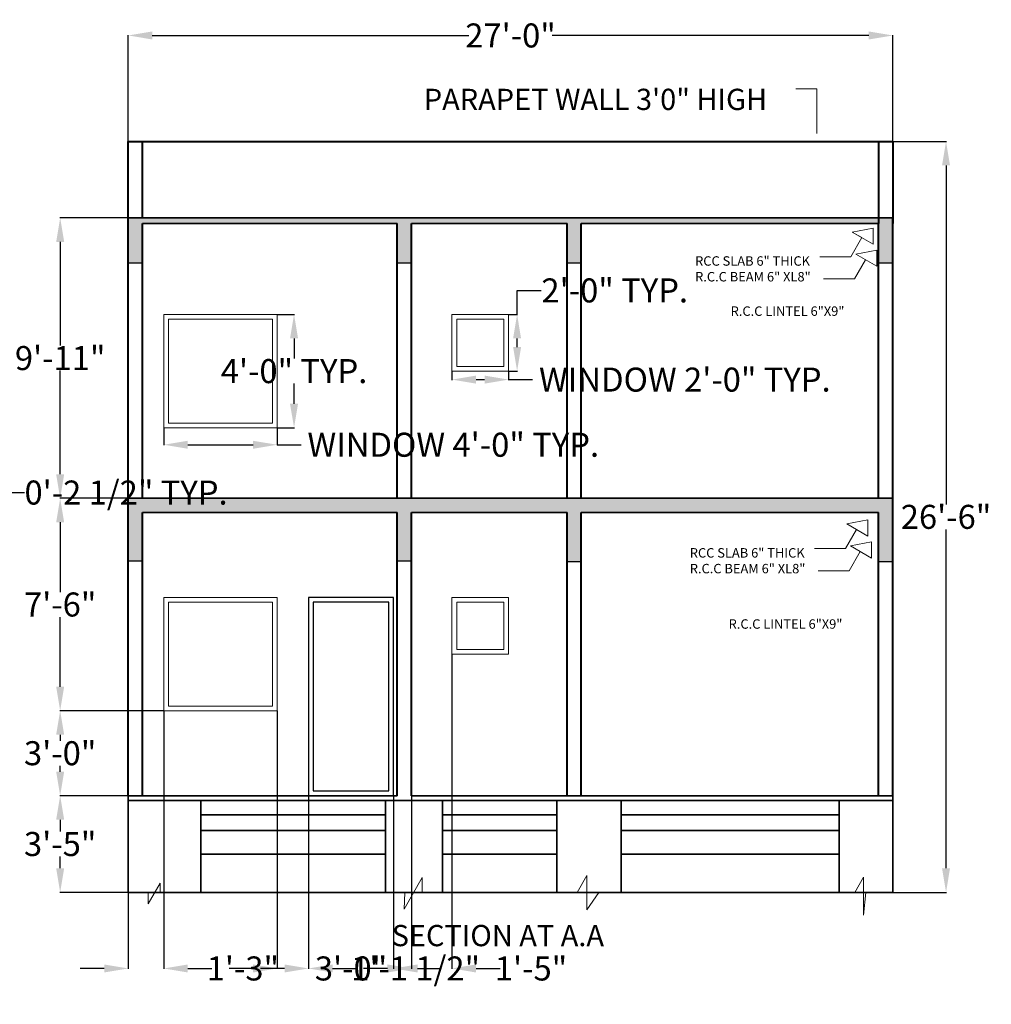
# Model space of a CAD drawing. Units: inches. Extents: x 2393 to 3270, y 740 to 1442.
# Tile 5 of 5: x 2823 to 3235, y 1024 to 1442. Entities that reach past the tile are written whole.
import ezdxf

# ---------------------------------------------------------------- set-up
doc = ezdxf.new("R2010")
doc.units = ezdxf.units.IN
doc.header["$MEASUREMENT"] = 0
for name, color, linetype, lineweight in [('A-ANNO-DIMS', 2, 'Continuous', 18), ('A-ANNO-SYMB', 3, 'Continuous', 18), ('A-ANNO-TEXT', 7, 'Continuous', 18), ('A-ANNO-TITL', 7, 'Continuous', 25), ('A-DOOR', 3, 'Continuous', 25), ('A-GLAZ', 4, 'Continuous', 18), ('A-SECT', 7, 'Continuous', 40), ('S-BEAM', 1, 'Continuous', 30), ('S-FNDN', 1, 'Continuous', 35), ('S-SLAB', 2, 'Continuous', 35)]:
    doc.layers.add(name, color=color, linetype=linetype, lineweight=lineweight)
doc.layers.add('S-CONC-PATT', color=18, linetype='Continuous', lineweight=13, true_color=0x000000)
doc.styles.get("Standard").update_dxf_attribs({"font": 'arial.ttf'})
doc.dimstyles.get("Standard").update_dxf_attribs({"dimtxt": 10.18, "dimasz": 10.18, "dimexe": 0.18, "dimexo": 0.0625, "dimgap": 0.09, "dimtad": 0, "dimtih": 1, "dimtoh": 1, "dimdec": 0, "dimzin": 0, "dimdsep": 46, "dimlunit": 3, "dimtxsty": 'Standard', "dimcen": 0.09, "dimadec": 0, "dimazin": 0, "dimtfac": 1, "dimtdec": 0, "dimtofl": 0, "dimtmove": 0, "dimatfit": 3, "dimfxl": 1, "dimtolj": 1, "dimtzin": 0, "dimarcsym": 0})

# ---------------------------------------------------------------- blocks, each defined once
blk = doc.blocks.new('WIN-48-SECTION')
for points in [[(0, 0), (48, 0), (48, 48), (0, 48)], [(2, 2), (46, 2), (46, 46), (2, 46)]]:
    blk.add_lwpolyline(points, close=True)
blk = doc.blocks.new('WIN-24-SECTION')
for points in [[(0, 0), (24, 0), (24, 24), (0, 24)], [(2, 2), (22, 2), (22, 22), (2, 22)]]:
    blk.add_lwpolyline(points, close=True)
blk = doc.blocks.new('LEADER-RCC-SLAB')
for p, q in [((22.71, 12.19), (13.77, 10.46)), ((17.84, 8.11), (13.77, 10.46)), ((13.77, 10.46), (22.71, 5.3)), ((22.71, 5.3), (22.71, 12.19)), ((13.15, 0), (17.84, 8.11)), ((0, 0), (13.15, 0))]:
    blk.add_line(p, q)
blk = doc.blocks.new('LEADER-RCC-BEAM')
for p, q in [((22.71, 12.19), (13.77, 10.46)), ((13.77, 10.46), (22.71, 5.3)), ((22.71, 5.3), (22.71, 12.19)), ((13.15, 0), (17.84, 8.11)), ((0, 0), (13.15, 0))]:
    blk.add_line(p, q)
blk = doc.blocks.new('*D41')
at = {"layer": 'A-ANNO-DIMS', "color": 0, "lineweight": -2, "transparency": 16777216}
for p, q in [((2814.97, 1231.01), (2814.97, 1241.19)), ((2814.97, 1241.19), (2825.15, 1241.19)), ((2766.16, 1220.83), (2815.15, 1220.83)), ((2766.16, 1218.43), (2815.15, 1218.43)), ((2814.97, 1208.25), (2814.97, 1198.07))]:
    blk.add_line(p, q, dxfattribs=at)
at = {"layer": 'A-ANNO-DIMS', "color": 0, "transparency": 16777216}
for points in [[(2813.27, 1231.01), (2816.67, 1231.01), (2814.97, 1220.83)], [(2813.27, 1208.25), (2816.67, 1208.25), (2814.97, 1218.43)]]:
    blk.add_solid(points, dxfattribs=at)
at = {"layer": 'Defpoints', "color": 0, "transparency": 16777216}
for p in [(2766.1, 1220.83), (2766.1, 1218.43), (2814.97, 1220.83)]:
    blk.add_point(p, dxfattribs=at)
at = {"layer": 'A-ANNO-DIMS', "color": 0, "transparency": 16777216, "insert": (2868.13, 1241.19), "char_height": 10.18, "attachment_point": 5}
blk.add_mtext('\\A1;0\'-2 1/2" TYP.', dxfattribs=at)
blk = doc.blocks.new('*D42')
at = {"layer": 'A-ANNO-DIMS', "color": 0, "lineweight": -2, "transparency": 16777216}
for p, q in [((2884.13, 1268.57), (2884.13, 1261.26)), ((2932.13, 1268.57), (2932.13, 1261.26)), ((2894.31, 1261.44), (2921.95, 1261.44)), ((2932.13, 1261.44), (2942.31, 1261.44))]:
    blk.add_line(p, q, dxfattribs=at)
at = {"layer": 'A-ANNO-DIMS', "color": 0, "transparency": 16777216}
for points in [[(2894.31, 1263.13), (2894.31, 1259.74), (2884.13, 1261.44)], [(2921.95, 1263.13), (2921.95, 1259.74), (2932.13, 1261.44)]]:
    blk.add_solid(points, dxfattribs=at)
at = {"layer": 'Defpoints', "color": 0, "transparency": 16777216}
for p in [(2884.13, 1268.64), (2932.13, 1268.64), (2932.13, 1261.44)]:
    blk.add_point(p, dxfattribs=at)
at = {"layer": 'A-ANNO-DIMS', "color": 0, "transparency": 16777216, "insert": (3006.81, 1261.44), "char_height": 10.18, "attachment_point": 5}
blk.add_mtext('\\A1;WINDOW 4\'-0" TYP.', dxfattribs=at)
blk = doc.blocks.new('*D43')
at = {"layer": 'A-ANNO-DIMS', "color": 0, "lineweight": -2, "transparency": 16777216}
for p, q in [((2932.19, 1316.64), (2939.51, 1316.64)), ((2939.33, 1306.46), (2939.33, 1297.92)), ((2939.33, 1278.82), (2939.33, 1287.35)), ((2932.19, 1268.64), (2939.51, 1268.64))]:
    blk.add_line(p, q, dxfattribs=at)
at = {"layer": 'A-ANNO-DIMS', "color": 0, "transparency": 16777216}
for points in [[(2937.63, 1306.46), (2941.03, 1306.46), (2939.33, 1316.64)], [(2937.63, 1278.82), (2941.03, 1278.82), (2939.33, 1268.64)]]:
    blk.add_solid(points, dxfattribs=at)
at = {"layer": 'Defpoints', "color": 0, "transparency": 16777216}
for p in [(2932.13, 1316.64), (2939.33, 1316.64), (2932.13, 1268.64)]:
    blk.add_point(p, dxfattribs=at)
at = {"layer": 'A-ANNO-DIMS', "color": 0, "transparency": 16777216, "insert": (2939.33, 1292.64), "char_height": 10.18, "attachment_point": 5}
blk.add_mtext('\\A1;4\'-0" TYP.', dxfattribs=at)
blk = doc.blocks.new('*D44')
at = {"layer": 'A-ANNO-DIMS', "color": 0, "lineweight": -2, "transparency": 16777216}
for p, q in [((3006.27, 1292.57), (3006.27, 1288.86)), ((3016.45, 1289.04), (3020.09, 1289.04)), ((3030.27, 1292.57), (3030.27, 1288.86)), ((3030.27, 1289.04), (3040.45, 1289.04))]:
    blk.add_line(p, q, dxfattribs=at)
at = {"layer": 'A-ANNO-DIMS', "color": 0, "transparency": 16777216}
for points in [[(3016.45, 1290.73), (3016.45, 1287.34), (3006.27, 1289.04)], [(3020.09, 1290.73), (3020.09, 1287.34), (3030.27, 1289.04)]]:
    blk.add_solid(points, dxfattribs=at)
at = {"layer": 'Defpoints', "color": 0, "transparency": 16777216}
for p in [(3006.27, 1292.64), (3030.27, 1292.64), (3030.27, 1289.04)]:
    blk.add_point(p, dxfattribs=at)
at = {"layer": 'A-ANNO-DIMS', "color": 0, "transparency": 16777216, "insert": (3104.95, 1289.04), "char_height": 10.18, "attachment_point": 5}
blk.add_mtext('\\A1;WINDOW 2\'-0" TYP.', dxfattribs=at)
blk = doc.blocks.new('*D45')
at = {"layer": 'A-ANNO-DIMS', "color": 0, "lineweight": -2, "transparency": 16777216}
for p, q in [((3033.87, 1316.64), (3033.87, 1326.82)), ((3033.87, 1326.82), (3044.05, 1326.82)), ((3030.33, 1316.64), (3034.05, 1316.64)), ((3033.87, 1302.82), (3033.87, 1306.46)), ((3030.33, 1292.64), (3034.05, 1292.64))]:
    blk.add_line(p, q, dxfattribs=at)
at = {"layer": 'A-ANNO-DIMS', "color": 0, "transparency": 16777216}
for points in [[(3032.17, 1306.46), (3035.56, 1306.46), (3033.87, 1316.64)], [(3032.17, 1302.82), (3035.56, 1302.82), (3033.87, 1292.64)]]:
    blk.add_solid(points, dxfattribs=at)
at = {"layer": 'Defpoints', "color": 0, "transparency": 16777216}
for p in [(3030.27, 1316.64), (3033.87, 1316.64), (3030.27, 1292.64)]:
    blk.add_point(p, dxfattribs=at)
at = {"layer": 'A-ANNO-DIMS', "color": 0, "transparency": 16777216, "insert": (3075.25, 1326.82), "char_height": 10.18, "attachment_point": 5}
blk.add_mtext('\\A1;2\'-0" TYP.', dxfattribs=at)
blk = doc.blocks.new('*D74')
at = {"layer": 'A-ANNO-DIMS', "color": 0, "lineweight": -2, "transparency": 16777216}
for p, q in [((2869.08, 1390.01), (2869.08, 1435.01)), ((3193.08, 1390.01), (3193.08, 1435.01)), ((2879.26, 1434.83), (3013.42, 1434.83)), ((3182.9, 1434.83), (3048.74, 1434.83))]:
    blk.add_line(p, q, dxfattribs=at)
at = {"layer": 'A-ANNO-DIMS', "color": 0, "transparency": 16777216}
for points in [[(2879.26, 1436.53), (2879.26, 1433.13), (2869.08, 1434.83)], [(3182.9, 1436.53), (3182.9, 1433.13), (3193.08, 1434.83)]]:
    blk.add_solid(points, dxfattribs=at)
at = {"layer": 'Defpoints', "color": 0, "transparency": 16777216}
for p in [(3193.08, 1434.83), (2869.08, 1389.95), (3193.08, 1389.95)]:
    blk.add_point(p, dxfattribs=at)
at = {"layer": 'A-ANNO-DIMS', "color": 0, "transparency": 16777216, "insert": (3031.08, 1434.83), "char_height": 10.18, "attachment_point": 5}
blk.add_mtext('\\A1;27\'-0"', dxfattribs=at)
blk = doc.blocks.new('*D75')
at = {"layer": 'A-ANNO-DIMS', "color": 0, "lineweight": -2, "transparency": 16777216}
for p, q in [((3193.14, 1389.95), (3215.84, 1389.95)), ((3215.66, 1379.77), (3215.66, 1236.18)), ((3215.66, 1082.01), (3215.66, 1225.6)), ((3193.14, 1071.83), (3215.84, 1071.83))]:
    blk.add_line(p, q, dxfattribs=at)
at = {"layer": 'A-ANNO-DIMS', "color": 0, "transparency": 16777216}
for points in [[(3213.96, 1379.77), (3217.35, 1379.77), (3215.66, 1389.95)], [(3213.96, 1082.01), (3217.35, 1082.01), (3215.66, 1071.83)]]:
    blk.add_solid(points, dxfattribs=at)
at = {"layer": 'Defpoints', "color": 0, "transparency": 16777216}
for p in [(3193.08, 1389.95), (3215.66, 1389.95), (3193.08, 1071.83)]:
    blk.add_point(p, dxfattribs=at)
at = {"layer": 'A-ANNO-DIMS', "color": 0, "transparency": 16777216, "insert": (3215.66, 1230.89), "char_height": 10.18, "attachment_point": 5}
blk.add_mtext('\\A1;26\'-6"', dxfattribs=at)
blk = doc.blocks.new('*D76')
at = {"layer": 'A-ANNO-DIMS', "color": 0, "lineweight": -2, "transparency": 16777216}
for p, q in [((2869.02, 1112.76), (2840.03, 1112.76)), ((2840.21, 1102.58), (2840.21, 1097.59)), ((2840.21, 1082.01), (2840.21, 1087.01)), ((2869.02, 1071.83), (2840.03, 1071.83))]:
    blk.add_line(p, q, dxfattribs=at)
at = {"layer": 'A-ANNO-DIMS', "color": 0, "transparency": 16777216}
for points in [[(2838.51, 1102.58), (2841.91, 1102.58), (2840.21, 1112.76)], [(2838.51, 1082.01), (2841.91, 1082.01), (2840.21, 1071.83)]]:
    blk.add_solid(points, dxfattribs=at)
at = {"layer": 'Defpoints', "color": 0, "transparency": 16777216}
for p in [(2840.21, 1112.76), (2869.08, 1112.76), (2869.08, 1071.83)]:
    blk.add_point(p, dxfattribs=at)
at = {"layer": 'A-ANNO-DIMS', "color": 0, "transparency": 16777216, "insert": (2840.21, 1092.3), "char_height": 10.18, "attachment_point": 5}
blk.add_mtext('\\A1;3\'-5"', dxfattribs=at)
blk = doc.blocks.new('*D77')
at = {"layer": 'A-ANNO-DIMS', "color": 0, "lineweight": -2, "transparency": 16777216}
for p, q in [((2884.07, 1148.76), (2840.03, 1148.76)), ((2840.21, 1138.58), (2840.21, 1136.05)), ((2840.21, 1122.94), (2840.21, 1125.47)), ((2869.02, 1112.76), (2840.03, 1112.76))]:
    blk.add_line(p, q, dxfattribs=at)
at = {"layer": 'A-ANNO-DIMS', "color": 0, "transparency": 16777216}
for points in [[(2838.51, 1138.58), (2841.91, 1138.58), (2840.21, 1148.76)], [(2838.51, 1122.94), (2841.91, 1122.94), (2840.21, 1112.76)]]:
    blk.add_solid(points, dxfattribs=at)
at = {"layer": 'Defpoints', "color": 0, "transparency": 16777216}
for p in [(2840.21, 1148.76), (2884.13, 1148.76), (2869.08, 1112.76)]:
    blk.add_point(p, dxfattribs=at)
at = {"layer": 'A-ANNO-DIMS', "color": 0, "transparency": 16777216, "insert": (2840.21, 1130.76), "char_height": 10.18, "attachment_point": 5}
blk.add_mtext('\\A1;3\'-0"', dxfattribs=at)
blk = doc.blocks.new('*D78')
at = {"layer": 'A-ANNO-DIMS', "color": 0, "lineweight": -2, "transparency": 16777216}
for p, q in [((2869.02, 1238.76), (2840.03, 1238.76)), ((2840.21, 1228.58), (2840.21, 1199.05)), ((2840.21, 1158.94), (2840.21, 1188.47)), ((2884.07, 1148.76), (2840.03, 1148.76))]:
    blk.add_line(p, q, dxfattribs=at)
at = {"layer": 'A-ANNO-DIMS', "color": 0, "transparency": 16777216}
for points in [[(2838.51, 1228.58), (2841.91, 1228.58), (2840.21, 1238.76)], [(2838.51, 1158.94), (2841.91, 1158.94), (2840.21, 1148.76)]]:
    blk.add_solid(points, dxfattribs=at)
at = {"layer": 'Defpoints', "color": 0, "transparency": 16777216}
for p in [(2840.21, 1238.76), (2869.08, 1238.76), (2884.13, 1148.76)]:
    blk.add_point(p, dxfattribs=at)
at = {"layer": 'A-ANNO-DIMS', "color": 0, "transparency": 16777216, "insert": (2840.21, 1193.76), "char_height": 10.18, "attachment_point": 5}
blk.add_mtext('\\A1;7\'-6"', dxfattribs=at)
blk = doc.blocks.new('*D79')
at = {"layer": 'A-ANNO-DIMS', "color": 0, "lineweight": -2, "transparency": 16777216}
for p, q in [((2869.02, 1357.55), (2840.03, 1357.55)), ((2840.21, 1347.37), (2840.21, 1303.44)), ((2840.21, 1248.94), (2840.21, 1292.87)), ((2869.02, 1238.76), (2840.03, 1238.76))]:
    blk.add_line(p, q, dxfattribs=at)
at = {"layer": 'A-ANNO-DIMS', "color": 0, "transparency": 16777216}
for points in [[(2838.51, 1347.37), (2841.91, 1347.37), (2840.21, 1357.55)], [(2838.51, 1248.94), (2841.91, 1248.94), (2840.21, 1238.76)]]:
    blk.add_solid(points, dxfattribs=at)
at = {"layer": 'Defpoints', "color": 0, "transparency": 16777216}
for p in [(2840.21, 1357.55), (2869.08, 1357.55), (2869.08, 1238.76)]:
    blk.add_point(p, dxfattribs=at)
at = {"layer": 'A-ANNO-DIMS', "color": 0, "transparency": 16777216, "insert": (2840.21, 1298.16), "char_height": 10.18, "attachment_point": 5}
blk.add_mtext('\\A1;9\'-11"', dxfattribs=at)
blk = doc.blocks.new('*D80')
at = {"layer": 'A-ANNO-DIMS', "color": 0, "lineweight": -2, "transparency": 16777216}
for p, q in [((2884.13, 1148.7), (2884.13, 1039.4)), ((2869.08, 1112.7), (2869.08, 1039.4)), ((2858.9, 1039.58), (2848.72, 1039.58)), ((2894.31, 1039.58), (2904.49, 1039.58))]:
    blk.add_line(p, q, dxfattribs=at)
at = {"layer": 'A-ANNO-DIMS', "color": 0, "transparency": 16777216}
for points in [[(2858.9, 1041.27), (2858.9, 1037.88), (2869.08, 1039.58)], [(2894.31, 1041.27), (2894.31, 1037.88), (2884.13, 1039.58)]]:
    blk.add_solid(points, dxfattribs=at)
at = {"layer": 'Defpoints', "color": 0, "transparency": 16777216}
for p in [(2884.13, 1148.76), (2869.08, 1112.76), (2884.13, 1039.58)]:
    blk.add_point(p, dxfattribs=at)
at = {"layer": 'A-ANNO-DIMS', "color": 0, "transparency": 16777216, "insert": (2917.63, 1039.58), "char_height": 10.18, "attachment_point": 5}
blk.add_mtext('\\A1;1\'-3"', dxfattribs=at)
blk = doc.blocks.new('*D81')
at = {"layer": 'A-ANNO-DIMS', "color": 0, "lineweight": -2, "transparency": 16777216}
for p, q in [((2932.13, 1148.7), (2932.13, 1039.4)), ((2945.49, 1112.7), (2945.49, 1039.4)), ((2921.95, 1039.58), (2911.77, 1039.58)), ((2955.67, 1039.58), (2965.85, 1039.58))]:
    blk.add_line(p, q, dxfattribs=at)
at = {"layer": 'A-ANNO-DIMS', "color": 0, "transparency": 16777216}
for points in [[(2921.95, 1041.27), (2921.95, 1037.88), (2932.13, 1039.58)], [(2955.67, 1041.27), (2955.67, 1037.88), (2945.49, 1039.58)]]:
    blk.add_solid(points, dxfattribs=at)
at = {"layer": 'Defpoints', "color": 0, "transparency": 16777216}
for p in [(2932.13, 1148.76), (2945.49, 1112.76), (2945.49, 1039.58)]:
    blk.add_point(p, dxfattribs=at)
at = {"layer": 'A-ANNO-DIMS', "color": 0, "transparency": 16777216, "insert": (2990.86, 1039.58), "char_height": 10.18, "attachment_point": 5}
blk.add_mtext('\\A1;1\'-1 1/2"', dxfattribs=at)
blk = doc.blocks.new('*D82')
at = {"layer": 'A-ANNO-DIMS', "color": 0, "lineweight": -2, "transparency": 16777216}
for p, q in [((2945.49, 1112.7), (2945.49, 1039.4)), ((2981.49, 1112.7), (2981.49, 1039.4)), ((2935.31, 1039.58), (2925.13, 1039.58)), ((2991.67, 1039.58), (3001.85, 1039.58))]:
    blk.add_line(p, q, dxfattribs=at)
at = {"layer": 'A-ANNO-DIMS', "color": 0, "transparency": 16777216}
for points in [[(2935.31, 1041.27), (2935.31, 1037.88), (2945.49, 1039.58)], [(2991.67, 1041.27), (2991.67, 1037.88), (2981.49, 1039.58)]]:
    blk.add_solid(points, dxfattribs=at)
at = {"layer": 'Defpoints', "color": 0, "transparency": 16777216}
for p in [(2945.49, 1112.76), (2981.49, 1112.76), (2981.49, 1039.58)]:
    blk.add_point(p, dxfattribs=at)
at = {"layer": 'A-ANNO-DIMS', "color": 0, "transparency": 16777216, "insert": (2963.49, 1039.58), "char_height": 10.18, "attachment_point": 5}
blk.add_mtext('\\A1;3\'-0"', dxfattribs=at)
blk = doc.blocks.new('*D83')
at = {"layer": 'A-ANNO-DIMS', "color": 0, "lineweight": -2, "transparency": 16777216}
for p, q in [((3006.27, 1172.7), (3006.27, 1039.4)), ((2989.08, 1112.7), (2989.08, 1039.4)), ((2978.9, 1039.58), (2968.72, 1039.58)), ((3016.45, 1039.58), (3026.63, 1039.58))]:
    blk.add_line(p, q, dxfattribs=at)
at = {"layer": 'A-ANNO-DIMS', "color": 0, "transparency": 16777216}
for points in [[(2978.9, 1041.27), (2978.9, 1037.88), (2989.08, 1039.58)], [(3016.45, 1041.27), (3016.45, 1037.88), (3006.27, 1039.58)]]:
    blk.add_solid(points, dxfattribs=at)
at = {"layer": 'Defpoints', "color": 0, "transparency": 16777216}
for p in [(3006.27, 1172.76), (2989.08, 1112.76), (3006.27, 1039.58)]:
    blk.add_point(p, dxfattribs=at)
at = {"layer": 'A-ANNO-DIMS', "color": 0, "transparency": 16777216, "insert": (3039.77, 1039.58), "char_height": 10.18, "attachment_point": 5}
blk.add_mtext('\\A1;1\'-5"', dxfattribs=at)

msp = doc.modelspace()

# ---------------------------------------------------------------- hatches: boundary and pattern name
at = {"layer": 'S-CONC-PATT'}
h = msp.add_hatch(color=256, dxfattribs=at)
h.dxf.hatch_style = 1
h.paths.add_polyline_path([(2875.08, 1355.16), (2983.08, 1355.16), (2983.08, 1338.44), (2989.08, 1338.44), (2989.08, 1355.16), (3055.08, 1355.16), (3055.08, 1338.44), (3061.08, 1338.44), (3061.08, 1355.16), (3187.08, 1355.16), (3187.08, 1338.44), (3193.08, 1338.44), (3193.08, 1357.55), (2869.08, 1357.55), (2869.08, 1355.16), (2869.08, 1338.44), (2875.08, 1338.44)])
h = msp.add_hatch(color=256, dxfattribs=at)
h.dxf.hatch_style = 1
h.paths.add_polyline_path([(2869.08, 1238.76), (2869.08, 1232.76), (2869.08, 1212.33), (2875.08, 1212.33), (2875.08, 1232.76), (2983.08, 1232.76), (2983.08, 1212.29), (2989.08, 1212.29), (2989.08, 1232.76), (3055.08, 1232.76), (3055.08, 1211.94), (3061.08, 1211.94), (3061.08, 1232.76), (3187.08, 1232.76), (3187.08, 1211.94), (3193.08, 1211.94), (3193.08, 1232.76), (3193.08, 1238.76)])

# ---------------------------------------------------------------- linework, layer by layer
at = {"layer": 'A-ANNO-SYMB'}
for p, q in [((3152.02, 1412.25), (3160.96, 1412.25)), ((3160.96, 1412.25), (3160.96, 1393.25)), ((2985.95, 1064.69), (2993.69, 1078.1)), ((2993.69, 1078.1), (2993.69, 1071.83)), ((3059.34, 1071.83), (3063.47, 1079)), ((3063.47, 1079), (3063.47, 1064.45)), ((3176.94, 1071.83), (3180.63, 1078.21)), ((3180.63, 1078.21), (3180.63, 1062.15)), ((2877.52, 1066.94), (2882.59, 1075.72)), ((2882.59, 1075.72), (2882.59, 1071.83)), ((2862.78, 1071.83), (2877.52, 1071.83)), ((2877.52, 1071.83), (2877.52, 1066.94)), ((2978.1, 1071.83), (2986.3, 1071.83)), ((2986.3, 1071.83), (2985.95, 1064.69)), ((3050.69, 1071.83), (3059.34, 1071.83)), ((3063.47, 1064.45), (3068.45, 1071.83)), ((3170.32, 1071.83), (3176.94, 1071.83)), ((3180.63, 1062.15), (3181.7, 1071.83))]:
    msp.add_line(p, q, dxfattribs=at)
at = {"layer": 'A-DOOR'}
for p, q in [((2981.49, 1196.76), (2945.49, 1196.76)), ((2945.49, 1196.76), (2945.49, 1112.76)), ((2979.49, 1194.76), (2947.49, 1194.76)), ((2947.49, 1194.76), (2947.49, 1114.76)), ((2979.49, 1114.76), (2979.49, 1194.76)), ((2981.49, 1112.76), (2981.49, 1196.76)), ((2947.49, 1114.76), (2979.49, 1114.76)), ((2945.49, 1112.76), (2981.49, 1112.76))]:
    msp.add_line(p, q, dxfattribs=at)
at = {"layer": 'A-SECT'}
for p, q in [((2869.08, 1357.55), (2869.08, 1389.95)), ((2869.08, 1389.95), (3193.08, 1389.95)), ((2875.08, 1357.55), (2875.08, 1389.95)), ((3187.08, 1389.95), (3187.08, 1355.16)), ((3193.08, 1389.95), (3193.08, 1355.16)), ((2869.08, 1355.16), (2869.08, 1357.55)), ((3193.08, 1232.76), (3193.08, 1357.55)), ((2869.08, 1232.76), (2869.08, 1355.16)), ((2875.08, 1238.76), (2875.08, 1355.16)), ((2983.08, 1238.76), (2983.08, 1355.16)), ((2989.08, 1238.76), (2989.08, 1355.16)), ((3055.08, 1238.76), (3055.08, 1355.16)), ((3061.08, 1238.76), (3061.08, 1355.16)), ((3187.08, 1238.76), (3187.08, 1355.16)), ((2869.08, 1112.76), (2869.08, 1232.76)), ((2875.08, 1112.76), (2875.08, 1232.76)), ((2983.08, 1112.76), (2983.08, 1232.76)), ((2989.08, 1112.76), (2989.08, 1232.76)), ((3055.08, 1112.76), (3055.08, 1232.76)), ((3061.08, 1112.76), (3061.08, 1232.76)), ((3187.08, 1112.76), (3187.08, 1232.76)), ((3193.08, 1112.76), (3193.08, 1232.76))]:
    msp.add_line(p, q, dxfattribs=at)
at = {"layer": 'S-BEAM'}
for p, q in [((2869.08, 1338.44), (2875.08, 1338.44)), ((2983.08, 1338.44), (2989.08, 1338.44)), ((3055.08, 1338.44), (3061.08, 1338.44)), ((3187.08, 1338.44), (3193.08, 1338.44)), ((2869.08, 1212.33), (2875.08, 1212.33)), ((2983.08, 1212.29), (2983.08, 1212.29)), ((2983.08, 1212.29), (2989.08, 1212.29)), ((3055.08, 1211.94), (3061.08, 1211.94)), ((3187.08, 1211.94), (3193.08, 1211.94))]:
    msp.add_line(p, q, dxfattribs=at)
at = {"layer": 'S-FNDN'}
for p, q in [((2869.08, 1071.83), (2869.08, 1112.76)), ((2899.81, 1110.76), (2899.81, 1071.83)), ((2978.1, 1110.76), (2978.1, 1071.83)), ((3002.29, 1071.83), (3002.29, 1110.76)), ((3050.69, 1110.76), (3050.69, 1071.83)), ((3078.04, 1071.83), (3078.04, 1110.76)), ((3170.32, 1071.83), (3170.32, 1110.76)), ((3193.08, 1112.76), (3193.08, 1071.83)), ((3193.08, 1110.76), (3193.08, 1071.83)), ((2899.81, 1104.62), (2978.1, 1104.62)), ((3002.29, 1104.62), (3050.69, 1104.62)), ((3078.04, 1104.62), (3170.32, 1104.62)), ((2899.81, 1098), (2978.1, 1098)), ((3002.29, 1098), (3050.69, 1098)), ((3078.04, 1098), (3170.32, 1098)), ((2899.81, 1088.04), (2978.1, 1088.04)), ((3002.29, 1088.04), (3050.69, 1088.04)), ((3078.04, 1088.04), (3170.32, 1088.04)), ((2869.08, 1071.83), (3193.08, 1071.83)), ((2899.81, 1071.83), (2899.81, 1071.83)), ((2978.1, 1071.83), (3002.29, 1071.83)), ((3050.69, 1071.83), (3078.04, 1071.83)), ((3193.08, 1071.83), (3170.32, 1071.83))]:
    msp.add_line(p, q, dxfattribs=at)
at = {"layer": 'S-SLAB'}
for p, q in [((2869.08, 1357.55), (3193.08, 1357.55)), ((2875.08, 1355.16), (2983.08, 1355.16)), ((2989.08, 1355.16), (3055.08, 1355.16)), ((3061.08, 1355.16), (3187.08, 1355.16)), ((2869.08, 1238.76), (3193.08, 1238.76)), ((2875.08, 1232.76), (2983.08, 1232.76)), ((2989.08, 1232.76), (3055.08, 1232.76)), ((3061.08, 1232.76), (3187.08, 1232.76)), ((2869.08, 1112.76), (2983.08, 1112.76)), ((2869.08, 1110.76), (3193.08, 1110.76)), ((2945.49, 1112.76), (2926.9, 1112.76)), ((2989.08, 1112.76), (3193.08, 1112.76))]:
    msp.add_line(p, q, dxfattribs=at)

# ---------------------------------------------------------------- block references
at = {"layer": 'A-ANNO-SYMB'}
for name, p in [('LEADER-RCC-SLAB', (3162.13, 1341.06)), ('LEADER-RCC-BEAM', (3163.66, 1331.73)), ('LEADER-RCC-SLAB', (3159.87, 1217.42)), ('LEADER-RCC-BEAM', (3161.4, 1208.09))]:
    msp.add_blockref(name, p, dxfattribs=at)
at = {"layer": 'A-GLAZ'}
for name, p in [('WIN-48-SECTION', (2884.13, 1268.64)), ('WIN-24-SECTION', (3006.26, 1292.64)), ('WIN-48-SECTION', (2884.13, 1148.76)), ('WIN-24-SECTION', (3006.26, 1172.76))]:
    msp.add_blockref(name, p, dxfattribs=at)

# ---------------------------------------------------------------- texts
at = {"layer": 'A-ANNO-TEXT', "attachment_point": 1}
for s, width, insert, char_height in [('PARAPET WALL 3\'0" HIGH', 157.6873, (2994.33, 1412.25), 9), ('RCC SLAB 6" THICK \\PR.C.C BEAM 6" XL8"', 142.5336, (3109.31, 1341.29), 4), ('R.C.C LINTEL 6"X9"', 142.5336, (3124.38, 1320.04), 4), ('RCC SLAB 6" THICK \\PR.C.C BEAM 6" XL8"', 142.5336, (3107.05, 1217.64), 4), ('R.C.C LINTEL 6"X9"', 142.5336, (3123.52, 1187.5), 4)]:
    msp.add_mtext_dynamic_manual_height_columns(s, width=width, gutter_width=1, heights=[0], dxfattribs=dict(at, insert=insert, char_height=char_height))
at = {"layer": 'A-ANNO-TITL', "insert": (2980.71, 1058.01), "char_height": 9, "attachment_point": 1}
msp.add_mtext_dynamic_manual_height_columns('SECTION AT A.A', width=140.3126, gutter_width=1, heights=[0], dxfattribs=at)

# ---------------------------------------------------------------- dimensions: what is measured, and where the dimension line sits
at = {"layer": 'A-ANNO-DIMS'}
for base, p1, p2, picture, middle in [((3193.08, 1434.83), (2869.08, 1389.95), (3193.08, 1389.95), '*D74', (3031.08, 1434.83)), ((3006.27, 1039.58), (2989.08, 1112.76), (3006.27, 1172.76), '*D83', (3039.77, 1039.58)), ((2884.1299, 1039.5752), (2869.0819, 1112.7606), (2884.1299, 1148.7606), '*D80', (2917.6313, 1039.5752)), ((2945.49, 1039.58), (2932.13, 1148.76), (2945.49, 1112.76), '*D81', (2990.86, 1039.58)), ((2981.49, 1039.58), (2945.49, 1112.76), (2981.49, 1112.76), '*D82', (2963.49, 1039.58))]:
    dim = msp.add_linear_dim(base=base, p1=p1, p2=p2, dimstyle='Standard', override={"dimdec": 1, "dimlfac": 1, "dimrnd": 0, "dimzin": 1, "dimdsep": 46, "dimlunit": 4, "dimfrac": 2}, dxfattribs=at)
    dim.commit()
    dim.dimension.update_dxf_attribs({"geometry": picture, "text_midpoint": middle})
for base, p1, p2, picture, middle in [((3215.66, 1389.95), (3193.08, 1071.83), (3193.08, 1389.95), '*D75', (3215.66, 1230.89)), ((2840.21, 1357.55), (2869.08, 1238.76), (2869.08, 1357.55), '*D79', (2840.21, 1298.16)), ((2840.21, 1238.76), (2884.13, 1148.76), (2869.08, 1238.76), '*D78', (2840.21, 1193.76)), ((2840.21, 1148.76), (2869.08, 1112.76), (2884.13, 1148.76), '*D77', (2840.21, 1130.76)), ((2840.21, 1112.76), (2869.08, 1071.83), (2869.08, 1112.76), '*D76', (2840.21, 1092.3))]:
    dim = msp.add_linear_dim(base=base, p1=p1, p2=p2, angle=90, dimstyle='Standard', override={"dimdec": 1, "dimlfac": 1, "dimrnd": 0, "dimzin": 1, "dimdsep": 46, "dimlunit": 4, "dimfrac": 2}, dxfattribs=at)
    dim.commit()
    dim.dimension.update_dxf_attribs({"geometry": picture, "text_midpoint": middle})
for base, p1, p2, picture, middle in [((3033.87, 1316.64), (3030.27, 1292.64), (3030.27, 1316.64), '*D45', (3075.25, 1326.82)), ((2939.33, 1316.64), (2932.13, 1268.64), (2932.13, 1316.64), '*D43', (2939.33, 1292.64)), ((2814.97, 1220.83), (2766.1, 1218.43), (2766.1, 1220.83), '*D41', (2868.13, 1241.19))]:
    dim = msp.add_linear_dim(base=base, p1=p1, p2=p2, angle=90, text='<> TYP.', dimstyle='Standard', override={"dimdec": 1, "dimlfac": 1, "dimrnd": 0, "dimzin": 1, "dimdsep": 46, "dimlunit": 4, "dimfrac": 2}, dxfattribs=at)
    dim.commit()
    dim.dimension.update_dxf_attribs({"geometry": picture, "text_midpoint": middle})
for base, p1, p2, picture, middle in [((3030.27, 1289.04), (3006.27, 1292.64), (3030.27, 1292.64), '*D44', (3104.95, 1289.04)), ((2932.13, 1261.44), (2884.13, 1268.64), (2932.13, 1268.64), '*D42', (3006.81, 1261.44))]:
    dim = msp.add_linear_dim(base=base, p1=p1, p2=p2, text='WINDOW <> TYP.', dimstyle='Standard', override={"dimdec": 1, "dimlfac": 1, "dimrnd": 0, "dimzin": 1, "dimdsep": 46, "dimlunit": 4, "dimfrac": 2}, dxfattribs=at)
    dim.commit()
    dim.dimension.update_dxf_attribs({"geometry": picture, "text_midpoint": middle})

doc.saveas('drawing.dxf')
